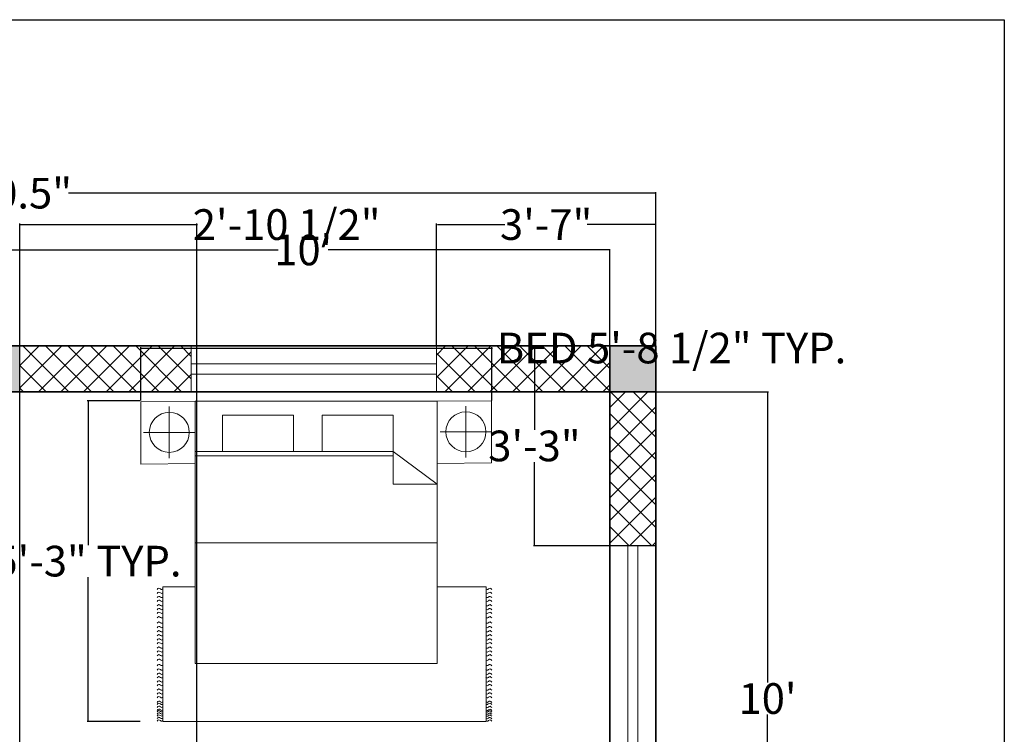
# Model space of a CAD drawing. Units: inches. Extents: x 958 to 1375, y 3152 to 3689.
# Tile 8 of 8: x 1182 to 1375, y 3550 to 3689. Entities that reach past the tile are written whole.
import ezdxf

# ---------------------------------------------------------------- set-up
doc = ezdxf.new("R2010")
doc.units = ezdxf.units.IN
doc.header["$MEASUREMENT"] = 0
for name, color, linetype, lineweight in [('A-ANNO-DIMS', 2, 'Continuous', 18), ('A-ANNO-TTLB', 7, 'Continuous', 25), ('A-FURN', 8, 'Continuous', 18), ('A-WALL', 7, 'Continuous', 35), ('windows', 140, 'Continuous', 18)]:
    doc.layers.add(name, color=color, linetype=linetype, lineweight=lineweight)
doc.layers.add('A-COLS-PATT', color=18, linetype='Continuous', lineweight=13, true_color=0x000000)
doc.layers.add('A-WALL-PATT', color=240, linetype='Continuous', lineweight=13, true_color=0xed1f24)
doc.styles.get("Standard").update_dxf_attribs({"font": 'arial.ttf'})
doc.dimstyles.get("Standard").update_dxf_attribs({"dimtxt": 6, "dimasz": 0.18, "dimexe": 0.18, "dimexo": 0.0625, "dimgap": 0.09, "dimtad": 0, "dimtih": 1, "dimtoh": 1, "dimdec": 1, "dimzin": 0, "dimdsep": 46, "dimlunit": 3, "dimtxsty": 'Standard', "dimcen": 0.09, "dimadec": 0, "dimazin": 0, "dimtfac": 1, "dimtdec": 1, "dimtofl": 0, "dimtmove": 0, "dimatfit": 3, "dimfxl": 1, "dimtolj": 1, "dimtzin": 0, "dimarcsym": 0})

# ---------------------------------------------------------------- blocks, each defined once
blk = doc.blocks.new('*D4')
at = {"layer": 'A-ANNO-DIMS', "color": 0, "lineweight": -2, "transparency": 16777216}
for p, q in [((1177.7, 3625.6), (1177.7, 3644.49)), ((1177.88, 3644.31), (1232.8, 3644.31)), ((1297.52, 3644.31), (1242.6, 3644.31)), ((1297.7, 3625.6), (1297.7, 3644.49))]:
    blk.add_line(p, q, dxfattribs=at)
at = {"layer": 'A-ANNO-DIMS', "color": 0, "transparency": 16777216}
for points in [[(1177.88, 3644.34), (1177.88, 3644.28), (1177.7, 3644.31)], [(1297.52, 3644.34), (1297.52, 3644.28), (1297.7, 3644.31)]]:
    blk.add_solid(points, dxfattribs=at)
at = {"layer": 'Defpoints', "color": 0, "transparency": 16777216}
for p in [(1297.7, 3644.31), (1177.7, 3625.53), (1297.7, 3625.53)]:
    blk.add_point(p, dxfattribs=at)
at = {"layer": 'A-ANNO-DIMS', "color": 0, "transparency": 16777216, "insert": (1237.7, 3644.31), "char_height": 6, "attachment_point": 5}
blk.add_mtext("\\A1;10'", dxfattribs=at)
blk = doc.blocks.new('*D5')
at = {"layer": 'A-ANNO-DIMS', "color": 0, "lineweight": -2, "transparency": 16777216}
for p, q in [((1306.76, 3616.53), (1328.75, 3616.53)), ((1328.57, 3616.35), (1328.57, 3559.69)), ((1328.57, 3496.71), (1328.57, 3553.38)), ((1306.76, 3496.53), (1328.75, 3496.53))]:
    blk.add_line(p, q, dxfattribs=at)
at = {"layer": 'A-ANNO-DIMS', "color": 0, "transparency": 16777216}
for points in [[(1328.54, 3616.35), (1328.6, 3616.35), (1328.57, 3616.53)], [(1328.54, 3496.71), (1328.6, 3496.71), (1328.57, 3496.53)]]:
    blk.add_solid(points, dxfattribs=at)
at = {"layer": 'Defpoints', "color": 0, "transparency": 16777216}
for p in [(1306.7, 3616.53), (1306.7, 3496.53), (1328.57, 3496.53)]:
    blk.add_point(p, dxfattribs=at)
at = {"layer": 'A-ANNO-DIMS', "color": 0, "transparency": 16777216, "insert": (1328.57, 3556.53), "char_height": 6, "attachment_point": 5}
blk.add_mtext("\\A1;10'", dxfattribs=at)
blk = doc.blocks.new('*D11')
at = {"layer": 'A-ANNO-DIMS', "color": 0, "lineweight": -2, "transparency": 16777216}
for p, q in [((1044.2, 3625.6), (1044.2, 3655.6)), ((1044.38, 3655.42), (1159.17, 3655.42)), ((1306.52, 3655.42), (1191.72, 3655.42)), ((1306.7, 3625.6), (1306.7, 3655.6))]:
    blk.add_line(p, q, dxfattribs=at)
at = {"layer": 'A-ANNO-DIMS', "color": 0, "transparency": 16777216}
for points in [[(1044.38, 3655.45), (1044.38, 3655.39), (1044.2, 3655.42)], [(1306.52, 3655.45), (1306.52, 3655.39), (1306.7, 3655.42)]]:
    blk.add_solid(points, dxfattribs=at)
at = {"layer": 'Defpoints', "color": 0, "transparency": 16777216}
for p in [(1306.7, 3655.42), (1044.2, 3625.53), (1306.7, 3625.53)]:
    blk.add_point(p, dxfattribs=at)
at = {"layer": 'A-ANNO-DIMS', "color": 0, "transparency": 16777216, "insert": (1175.45, 3655.42), "char_height": 6, "attachment_point": 5}
blk.add_mtext('\\A1;21\'-10.5"', dxfattribs=at)
blk = doc.blocks.new('BED-DOUBLE')
for p, q in [((63.65, 61.72), (63.65, 51.66)), ((5.6, 61.62), (5.6, 51.56)), ((10.63, 56.59), (0.57, 56.59)), ((68.68, 56.69), (58.62, 56.69)), ((49.39, 52.82), (10.63, 52.82)), ((49.39, 52.82), (58, 46.47)), ((49.44, 52.82), (49.44, 46.47)), ((49.44, 52), (10.63, 52)), ((49.44, 46.47), (58, 46.47)), ((58.05, 34.96), (10.63, 34.96)), ((4.36, 0), (4.36, 26.37)), ((4.36, 26.37), (10.65, 26.37)), ((58.05, 26.37), (67.59, 26.37)), ((67.59, 26.37), (67.59, 0)), ((67.59, 0), (4.36, 0))]:
    blk.add_line(p, q)
for points in [[(0, 50.39), (10.63, 50.5), (10.63, 62.68), (0, 62.58)], [(58.05, 62.68), (58.05, 11.37), (10.63, 11.37), (10.63, 62.68)], [(58.05, 50.5), (68.68, 50.6), (68.68, 62.78), (58.05, 62.68)], [(29.88, 59.98), (29.88, 52.82), (15.98, 52.82), (15.98, 59.98)], [(49.44, 59.98), (49.44, 52.82), (35.55, 52.82), (35.55, 59.98)]]:
    blk.add_lwpolyline(points, close=True)
for centre in [(5.6, 56.59), (63.65, 56.69)]:
    blk.add_circle(centre, 3.92)
for points, knots in [([(3.23, 25.84), (3.32, 25.96), (3.52, 26.2), (3.86, 25.96), (4.14, 25.78), (4.29, 25.89), (4.36, 25.94)], [0, 0, 0, 0, 0.400747, 0.791423, 1.067667, 1.29709, 1.29709, 1.29709, 1.29709]), ([(3.23, 25.06), (3.32, 25.18), (3.52, 25.42), (3.86, 25.18), (4.14, 25.01), (4.29, 25.11), (4.36, 25.16)], [0, 0, 0, 0, 0.400747, 0.791423, 1.067667, 1.29709, 1.29709, 1.29709, 1.29709]), ([(68.71, 25.84), (68.61, 25.96), (68.42, 26.2), (68.08, 25.96), (67.8, 25.78), (67.65, 25.89), (67.58, 25.94)], [0, 0, 0, 0, 0.400747, 0.791423, 1.067667, 1.29709, 1.29709, 1.29709, 1.29709]), ([(68.71, 25.06), (68.61, 25.18), (68.42, 25.42), (68.08, 25.18), (67.8, 25.01), (67.65, 25.11), (67.58, 25.16)], [0, 0, 0, 0, 0.400747, 0.791423, 1.067667, 1.29709, 1.29709, 1.29709, 1.29709]), ([(3.23, 24.24), (3.32, 24.36), (3.52, 24.6), (3.86, 24.36), (4.14, 24.19), (4.29, 24.3), (4.36, 24.34)], [0, 0, 0, 0, 0.400747, 0.791423, 1.067667, 1.29709, 1.29709, 1.29709, 1.29709]), ([(3.23, 23.51), (3.32, 23.63), (3.52, 23.87), (3.86, 23.63), (4.14, 23.46), (4.29, 23.57), (4.36, 23.62)], [0, 0, 0, 0, 0.400747, 0.791423, 1.067667, 1.29709, 1.29709, 1.29709, 1.29709]), ([(68.71, 24.24), (68.61, 24.36), (68.42, 24.6), (68.08, 24.36), (67.8, 24.19), (67.65, 24.3), (67.58, 24.34)], [0, 0, 0, 0, 0.400747, 0.791423, 1.067667, 1.29709, 1.29709, 1.29709, 1.29709]), ([(68.71, 23.51), (68.61, 23.63), (68.42, 23.87), (68.08, 23.63), (67.8, 23.46), (67.65, 23.57), (67.58, 23.62)], [0, 0, 0, 0, 0.400747, 0.791423, 1.067667, 1.29709, 1.29709, 1.29709, 1.29709]), ([(3.23, 22.63), (3.32, 22.75), (3.52, 22.99), (3.86, 22.75), (4.14, 22.58), (4.29, 22.69), (4.36, 22.73)], [0, 0, 0, 0, 0.400747, 0.791423, 1.067667, 1.29709, 1.29709, 1.29709, 1.29709]), ([(3.23, 21.88), (3.32, 22), (3.52, 22.24), (3.86, 22), (4.14, 21.83), (4.29, 21.93), (4.36, 21.98)], [0, 0, 0, 0, 0.400747, 0.791423, 1.067667, 1.29709, 1.29709, 1.29709, 1.29709]), ([(3.23, 21.15), (3.32, 21.27), (3.52, 21.51), (3.86, 21.27), (4.14, 21.1), (4.29, 21.21), (4.36, 21.25)], [0, 0, 0, 0, 0.400747, 0.791423, 1.067667, 1.29709, 1.29709, 1.29709, 1.29709]), ([(68.71, 22.63), (68.61, 22.75), (68.42, 22.99), (68.08, 22.75), (67.8, 22.58), (67.65, 22.69), (67.58, 22.73)], [0, 0, 0, 0, 0.400747, 0.791423, 1.067667, 1.29709, 1.29709, 1.29709, 1.29709]), ([(68.71, 21.88), (68.61, 22), (68.42, 22.24), (68.08, 22), (67.8, 21.83), (67.65, 21.93), (67.58, 21.98)], [0, 0, 0, 0, 0.400747, 0.791423, 1.067667, 1.29709, 1.29709, 1.29709, 1.29709]), ([(68.71, 21.15), (68.61, 21.27), (68.42, 21.51), (68.08, 21.27), (67.8, 21.1), (67.65, 21.21), (67.58, 21.25)], [0, 0, 0, 0, 0.400747, 0.791423, 1.067667, 1.29709, 1.29709, 1.29709, 1.29709]), ([(3.23, 20.27), (3.32, 20.39), (3.52, 20.63), (3.86, 20.39), (4.14, 20.22), (4.29, 20.32), (4.36, 20.37)], [0, 0, 0, 0, 0.400747, 0.791423, 1.067667, 1.29709, 1.29709, 1.29709, 1.29709]), ([(3.23, 19.23), (3.32, 19.35), (3.52, 19.59), (3.86, 19.35), (4.14, 19.18), (4.29, 19.29), (4.36, 19.33)], [0, 0, 0, 0, 0.400747, 0.791423, 1.067667, 1.29709, 1.29709, 1.29709, 1.29709]), ([(68.71, 20.27), (68.61, 20.39), (68.42, 20.63), (68.08, 20.39), (67.8, 20.22), (67.65, 20.32), (67.58, 20.37)], [0, 0, 0, 0, 0.400747, 0.791423, 1.067667, 1.29709, 1.29709, 1.29709, 1.29709]), ([(68.71, 19.23), (68.61, 19.35), (68.42, 19.59), (68.08, 19.35), (67.8, 19.18), (67.65, 19.29), (67.58, 19.33)], [0, 0, 0, 0, 0.400747, 0.791423, 1.067667, 1.29709, 1.29709, 1.29709, 1.29709]), ([(3.23, 18.35), (3.32, 18.47), (3.52, 18.71), (3.86, 18.47), (4.14, 18.3), (4.29, 18.4), (4.36, 18.45)], [0, 0, 0, 0, 0.400747, 0.791423, 1.067667, 1.29709, 1.29709, 1.29709, 1.29709]), ([(3.23, 17.53), (3.32, 17.65), (3.52, 17.89), (3.86, 17.65), (4.14, 17.48), (4.29, 17.59), (4.36, 17.64)], [0, 0, 0, 0, 0.400747, 0.791423, 1.067667, 1.29709, 1.29709, 1.29709, 1.29709]), ([(68.71, 18.35), (68.61, 18.47), (68.42, 18.71), (68.08, 18.47), (67.8, 18.3), (67.65, 18.4), (67.58, 18.45)], [0, 0, 0, 0, 0.400747, 0.791423, 1.067667, 1.29709, 1.29709, 1.29709, 1.29709]), ([(68.71, 17.53), (68.61, 17.65), (68.42, 17.89), (68.08, 17.65), (67.8, 17.48), (67.65, 17.59), (67.58, 17.64)], [0, 0, 0, 0, 0.400747, 0.791423, 1.067667, 1.29709, 1.29709, 1.29709, 1.29709]), ([(3.23, 16.76), (3.32, 16.88), (3.52, 17.12), (3.86, 16.88), (4.14, 16.71), (4.29, 16.81), (4.36, 16.86)], [0, 0, 0, 0, 0.400747, 0.791423, 1.067667, 1.29709, 1.29709, 1.29709, 1.29709]), ([(3.23, 15.94), (3.32, 16.06), (3.52, 16.3), (3.86, 16.06), (4.14, 15.89), (4.29, 16), (4.36, 16.04)], [0, 0, 0, 0, 0.400747, 0.791423, 1.067667, 1.29709, 1.29709, 1.29709, 1.29709]), ([(3.23, 15.21), (3.32, 15.33), (3.52, 15.57), (3.86, 15.33), (4.14, 15.16), (4.29, 15.27), (4.36, 15.32)], [0, 0, 0, 0, 0.400747, 0.791423, 1.067667, 1.29709, 1.29709, 1.29709, 1.29709]), ([(68.71, 16.76), (68.61, 16.88), (68.42, 17.12), (68.08, 16.88), (67.8, 16.71), (67.65, 16.81), (67.58, 16.86)], [0, 0, 0, 0, 0.400747, 0.791423, 1.067667, 1.29709, 1.29709, 1.29709, 1.29709]), ([(68.71, 15.94), (68.61, 16.06), (68.42, 16.3), (68.08, 16.06), (67.8, 15.89), (67.65, 16), (67.58, 16.04)], [0, 0, 0, 0, 0.400747, 0.791423, 1.067667, 1.29709, 1.29709, 1.29709, 1.29709]), ([(68.71, 15.21), (68.61, 15.33), (68.42, 15.57), (68.08, 15.33), (67.8, 15.16), (67.65, 15.27), (67.58, 15.32)], [0, 0, 0, 0, 0.400747, 0.791423, 1.067667, 1.29709, 1.29709, 1.29709, 1.29709]), ([(3.23, 14.33), (3.32, 14.45), (3.52, 14.69), (3.86, 14.45), (4.14, 14.28), (4.29, 14.39), (4.36, 14.43)], [0, 0, 0, 0, 0.400747, 0.791423, 1.067667, 1.29709, 1.29709, 1.29709, 1.29709]), ([(3.23, 13.58), (3.32, 13.7), (3.52, 13.94), (3.86, 13.7), (4.14, 13.53), (4.29, 13.63), (4.36, 13.68)], [0, 0, 0, 0, 0.400747, 0.791423, 1.067667, 1.29709, 1.29709, 1.29709, 1.29709]), ([(68.71, 14.33), (68.61, 14.45), (68.42, 14.69), (68.08, 14.45), (67.8, 14.28), (67.65, 14.39), (67.58, 14.43)], [0, 0, 0, 0, 0.400747, 0.791423, 1.067667, 1.29709, 1.29709, 1.29709, 1.29709]), ([(68.71, 13.58), (68.61, 13.7), (68.42, 13.94), (68.08, 13.7), (67.8, 13.53), (67.65, 13.63), (67.58, 13.68)], [0, 0, 0, 0, 0.400747, 0.791423, 1.067667, 1.29709, 1.29709, 1.29709, 1.29709]), ([(3.23, 12.85), (3.32, 12.97), (3.52, 13.21), (3.86, 12.97), (4.14, 12.8), (4.29, 12.9), (4.36, 12.95)], [0, 0, 0, 0, 0.400747, 0.791423, 1.067667, 1.29709, 1.29709, 1.29709, 1.29709]), ([(3.23, 11.97), (3.32, 12.09), (3.52, 12.33), (3.86, 12.09), (4.14, 11.92), (4.29, 12.02), (4.36, 12.07)], [0, 0, 0, 0, 0.400747, 0.791423, 1.067667, 1.29709, 1.29709, 1.29709, 1.29709]), ([(68.71, 12.85), (68.61, 12.97), (68.42, 13.21), (68.08, 12.97), (67.8, 12.8), (67.65, 12.9), (67.58, 12.95)], [0, 0, 0, 0, 0.400747, 0.791423, 1.067667, 1.29709, 1.29709, 1.29709, 1.29709]), ([(68.71, 11.97), (68.61, 12.09), (68.42, 12.33), (68.08, 12.09), (67.8, 11.92), (67.65, 12.02), (67.58, 12.07)], [0, 0, 0, 0, 0.400747, 0.791423, 1.067667, 1.29709, 1.29709, 1.29709, 1.29709]), ([(3.23, 10.93), (3.32, 11.05), (3.52, 11.29), (3.86, 11.05), (4.14, 10.88), (4.29, 10.99), (4.36, 11.03)], [0, 0, 0, 0, 0.400747, 0.791423, 1.067667, 1.29709, 1.29709, 1.29709, 1.29709]), ([(3.23, 10.05), (3.32, 10.17), (3.52, 10.41), (3.86, 10.17), (4.14, 10), (4.29, 10.1), (4.36, 10.15)], [0, 0, 0, 0, 0.400747, 0.791423, 1.067667, 1.29709, 1.29709, 1.29709, 1.29709]), ([(68.71, 10.93), (68.61, 11.05), (68.42, 11.29), (68.08, 11.05), (67.8, 10.88), (67.65, 10.99), (67.58, 11.03)], [0, 0, 0, 0, 0.400747, 0.791423, 1.067667, 1.29709, 1.29709, 1.29709, 1.29709]), ([(68.71, 10.05), (68.61, 10.17), (68.42, 10.41), (68.08, 10.17), (67.8, 10), (67.65, 10.1), (67.58, 10.15)], [0, 0, 0, 0, 0.400747, 0.791423, 1.067667, 1.29709, 1.29709, 1.29709, 1.29709]), ([(3.23, 9.23), (3.32, 9.35), (3.52, 9.59), (3.86, 9.35), (4.14, 9.18), (4.29, 9.29), (4.36, 9.34)], [0, 0, 0, 0, 0.400747, 0.791423, 1.067667, 1.29709, 1.29709, 1.29709, 1.29709]), ([(3.23, 8.54), (3.32, 8.66), (3.52, 8.9), (3.86, 8.66), (4.14, 8.49), (4.29, 8.6), (4.36, 8.65)], [0, 0, 0, 0, 0.400747, 0.791423, 1.067667, 1.29709, 1.29709, 1.29709, 1.29709]), ([(3.23, 7.73), (3.32, 7.85), (3.52, 8.09), (3.86, 7.85), (4.14, 7.68), (4.29, 7.78), (4.36, 7.83)], [0, 0, 0, 0, 0.400747, 0.791423, 1.067667, 1.29709, 1.29709, 1.29709, 1.29709]), ([(68.71, 9.23), (68.61, 9.35), (68.42, 9.59), (68.08, 9.35), (67.8, 9.18), (67.65, 9.29), (67.58, 9.34)], [0, 0, 0, 0, 0.400747, 0.791423, 1.067667, 1.29709, 1.29709, 1.29709, 1.29709]), ([(68.71, 8.54), (68.61, 8.66), (68.42, 8.9), (68.08, 8.66), (67.8, 8.49), (67.65, 8.6), (67.58, 8.65)], [0, 0, 0, 0, 0.400747, 0.791423, 1.067667, 1.29709, 1.29709, 1.29709, 1.29709]), ([(68.71, 7.73), (68.61, 7.85), (68.42, 8.09), (68.08, 7.85), (67.8, 7.68), (67.65, 7.78), (67.58, 7.83)], [0, 0, 0, 0, 0.400747, 0.791423, 1.067667, 1.29709, 1.29709, 1.29709, 1.29709]), ([(3.23, 7), (3.32, 7.12), (3.52, 7.36), (3.86, 7.12), (4.14, 6.95), (4.29, 7.05), (4.36, 7.1)], [0, 0, 0, 0, 0.400747, 0.791423, 1.067667, 1.29709, 1.29709, 1.29709, 1.29709]), ([(3.23, 6.12), (3.32, 6.24), (3.52, 6.48), (3.86, 6.24), (4.14, 6.07), (4.29, 6.17), (4.36, 6.22)], [0, 0, 0, 0, 0.400747, 0.791423, 1.067667, 1.29709, 1.29709, 1.29709, 1.29709]), ([(68.71, 7), (68.61, 7.12), (68.42, 7.36), (68.08, 7.12), (67.8, 6.95), (67.65, 7.05), (67.58, 7.1)], [0, 0, 0, 0, 0.400747, 0.791423, 1.067667, 1.29709, 1.29709, 1.29709, 1.29709]), ([(68.71, 6.12), (68.61, 6.24), (68.42, 6.48), (68.08, 6.24), (67.8, 6.07), (67.65, 6.17), (67.58, 6.22)], [0, 0, 0, 0, 0.400747, 0.791423, 1.067667, 1.29709, 1.29709, 1.29709, 1.29709]), ([(3.23, 5.37), (3.32, 5.49), (3.52, 5.73), (3.86, 5.49), (4.14, 5.31), (4.29, 5.42), (4.36, 5.47)], [0, 0, 0, 0, 0.400747, 0.791423, 1.067667, 1.29709, 1.29709, 1.29709, 1.29709]), ([(3.23, 4.64), (3.32, 4.76), (3.52, 5), (3.86, 4.76), (4.14, 4.59), (4.29, 4.69), (4.36, 4.74)], [0, 0, 0, 0, 0.400747, 0.791423, 1.067667, 1.29709, 1.29709, 1.29709, 1.29709]), ([(3.23, 3.75), (3.32, 3.88), (3.52, 4.12), (3.86, 3.88), (4.14, 3.7), (4.29, 3.81), (4.36, 3.86)], [0, 0, 0, 0, 0.400747, 0.791423, 1.067667, 1.29709, 1.29709, 1.29709, 1.29709]), ([(68.71, 5.37), (68.61, 5.49), (68.42, 5.73), (68.08, 5.49), (67.8, 5.31), (67.65, 5.42), (67.58, 5.47)], [0, 0, 0, 0, 0.400747, 0.791423, 1.067667, 1.29709, 1.29709, 1.29709, 1.29709]), ([(68.71, 4.64), (68.61, 4.76), (68.42, 5), (68.08, 4.76), (67.8, 4.59), (67.66, 4.69), (67.59, 4.73)], [0, 0, 0, 0, 0.400747, 0.791423, 1.067667, 1.283686, 1.283686, 1.283686, 1.283686]), ([(68.71, 3.75), (68.61, 3.88), (68.42, 4.12), (68.08, 3.88), (67.8, 3.7), (67.66, 3.81), (67.59, 3.85)], [0, 0, 0, 0, 0.400747, 0.791423, 1.067667, 1.283686, 1.283686, 1.283686, 1.283686]), ([(3.23, 3.33), (3.32, 3.45), (3.52, 3.7), (3.86, 3.45), (4.14, 3.27), (4.29, 3.38), (4.36, 3.43)], [0, 0, 0, 0, 0.407265, 0.802015, 1.07826, 1.307683, 1.307683, 1.307683, 1.307683]), ([(3.23, 2.76), (3.32, 2.88), (3.52, 3.12), (3.86, 2.88), (4.14, 2.71), (4.29, 2.81), (4.36, 2.86)], [0, 0, 0, 0, 0.400747, 0.791423, 1.067667, 1.29709, 1.29709, 1.29709, 1.29709]), ([(3.23, 2.19), (3.32, 2.31), (3.52, 2.55), (3.86, 2.31), (4.14, 2.13), (4.29, 2.24), (4.36, 2.29)], [0, 0, 0, 0, 0.400747, 0.791423, 1.067667, 1.29709, 1.29709, 1.29709, 1.29709]), ([(3.23, 1.88), (3.32, 2), (3.52, 2.24), (3.86, 2), (4.14, 1.82), (4.29, 1.93), (4.36, 1.98)], [0, 0, 0, 0, 0.400747, 0.791423, 1.067667, 1.29709, 1.29709, 1.29709, 1.29709]), ([(68.71, 3.33), (68.61, 3.45), (68.42, 3.69), (68.08, 3.45), (67.8, 3.28), (67.66, 3.38), (67.59, 3.42)], [0, 0, 0, 0, 0.402903, 0.794912, 1.071156, 1.287177, 1.287177, 1.287177, 1.287177]), ([(68.71, 2.73), (68.61, 2.85), (68.42, 3.09), (68.08, 2.85), (67.8, 2.68), (67.66, 2.78), (67.59, 2.83)], [0, 0, 0, 0, 0.400747, 0.791423, 1.067667, 1.283686, 1.283686, 1.283686, 1.283686]), ([(68.71, 2.16), (68.61, 2.28), (68.42, 2.52), (68.08, 2.28), (67.8, 2.11), (67.66, 2.21), (67.59, 2.25)], [0, 0, 0, 0, 0.400747, 0.791423, 1.067667, 1.283686, 1.283686, 1.283686, 1.283686]), ([(68.71, 1.85), (68.61, 1.97), (68.42, 2.21), (68.08, 1.97), (67.8, 1.8), (67.66, 1.9), (67.59, 1.94)], [0, 0, 0, 0, 0.400747, 0.791423, 1.067667, 1.283686, 1.283686, 1.283686, 1.283686]), ([(3.23, 1.46), (3.32, 1.58), (3.52, 1.82), (3.86, 1.58), (4.14, 1.41), (4.29, 1.51), (4.36, 1.56)], [0, 0, 0, 0, 0.400747, 0.791423, 1.067667, 1.29709, 1.29709, 1.29709, 1.29709]), ([(3.23, 1.06), (3.32, 1.18), (3.52, 1.42), (3.86, 1.18), (4.14, 1.01), (4.29, 1.11), (4.36, 1.16)], [0, 0, 0, 0, 0.400747, 0.791423, 1.067667, 1.29709, 1.29709, 1.29709, 1.29709]), ([(3.23, 0.57), (3.32, 0.7), (3.52, 0.94), (3.86, 0.7), (4.14, 0.52), (4.29, 0.63), (4.36, 0.68)], [0, 0, 0, 0, 0.400747, 0.791423, 1.067667, 1.29709, 1.29709, 1.29709, 1.29709]), ([(3.23, 0.07), (3.32, 0.19), (3.52, 0.43), (3.86, 0.19), (4.14, 0.02), (4.29, 0.13), (4.36, 0.18)], [0, 0, 0, 0, 0.400747, 0.791423, 1.067667, 1.29709, 1.29709, 1.29709, 1.29709]), ([(68.71, 1.43), (68.61, 1.55), (68.42, 1.79), (68.08, 1.55), (67.8, 1.38), (67.65, 1.48), (67.58, 1.53)], [0, 0, 0, 0, 0.400747, 0.791423, 1.067667, 1.29709, 1.29709, 1.29709, 1.29709]), ([(68.71, 1.03), (68.61, 1.15), (68.42, 1.39), (68.08, 1.15), (67.8, 0.98), (67.65, 1.09), (67.58, 1.13)], [0, 0, 0, 0, 0.400747, 0.791423, 1.067667, 1.29709, 1.29709, 1.29709, 1.29709]), ([(68.71, 0.55), (68.61, 0.67), (68.42, 0.91), (68.08, 0.67), (67.8, 0.5), (67.65, 0.6), (67.58, 0.65)], [0, 0, 0, 0, 0.400747, 0.791423, 1.067667, 1.29709, 1.29709, 1.29709, 1.29709]), ([(68.71, 0.07), (68.61, 0.19), (68.42, 0.43), (68.08, 0.19), (67.8, 0.02), (67.65, 0.13), (67.58, 0.18)], [0, 0, 0, 0, 0.400747, 0.791423, 1.067667, 1.29709, 1.29709, 1.29709, 1.29709])]:
    blk.add_open_spline(points, degree=3, knots=knots)
blk = doc.blocks.new('WIN-48')
for p, q in [((48, 9), (0, 9)), ((48, 5.5), (0, 5.5)), ((0, 3.5), (48, 3.5)), ((0, 0), (48, 0))]:
    blk.add_line(p, q)
blk = doc.blocks.new('*D26')
at = {"layer": 'A-ANNO-DIMS', "color": 0, "lineweight": -2, "transparency": 16777216}
for p, q in [((1205.88, 3614.87), (1205.88, 3625.3)), ((1206.06, 3625.12), (1274.41, 3625.12)), ((1274.59, 3614.87), (1274.59, 3625.3)), ((1274.59, 3625.12), (1274.77, 3625.12))]:
    blk.add_line(p, q, dxfattribs=at)
at = {"layer": 'A-ANNO-DIMS', "color": 0, "transparency": 16777216}
for points in [[(1206.06, 3625.15), (1206.06, 3625.09), (1205.88, 3625.12)], [(1274.41, 3625.15), (1274.41, 3625.09), (1274.59, 3625.12)]]:
    blk.add_solid(points, dxfattribs=at)
at = {"layer": 'Defpoints', "color": 0, "transparency": 16777216}
for p in [(1274.59, 3625.12), (1205.88, 3614.81), (1274.59, 3614.81)]:
    blk.add_point(p, dxfattribs=at)
at = {"layer": 'A-ANNO-DIMS', "color": 0, "transparency": 16777216, "insert": (1309.78, 3625.12), "char_height": 6, "attachment_point": 5}
blk.add_mtext('\\A1;BED 5\'-8 1/2" TYP.', dxfattribs=at)
blk = doc.blocks.new('*D27')
at = {"layer": 'A-ANNO-DIMS', "color": 0, "lineweight": -2, "transparency": 16777216}
for p, q in [((1205.81, 3614.81), (1195.39, 3614.81)), ((1195.57, 3614.63), (1195.57, 3586.57)), ((1195.57, 3552.21), (1195.57, 3580.26)), ((1205.81, 3552.03), (1195.39, 3552.03))]:
    blk.add_line(p, q, dxfattribs=at)
at = {"layer": 'A-ANNO-DIMS', "color": 0, "transparency": 16777216}
for points in [[(1195.54, 3614.63), (1195.6, 3614.63), (1195.57, 3614.81)], [(1195.54, 3552.21), (1195.6, 3552.21), (1195.57, 3552.03)]]:
    blk.add_solid(points, dxfattribs=at)
at = {"layer": 'Defpoints', "color": 0, "transparency": 16777216}
for p in [(1195.57, 3614.81), (1205.88, 3614.81), (1205.88, 3552.03)]:
    blk.add_point(p, dxfattribs=at)
at = {"layer": 'A-ANNO-DIMS', "color": 0, "transparency": 16777216, "insert": (1195.57, 3583.42), "char_height": 6, "attachment_point": 5}
blk.add_mtext('\\A1;5\'-3" TYP.', dxfattribs=at)
blk = doc.blocks.new('*D47')
at = {"layer": 'A-ANNO-DIMS', "color": 0, "lineweight": -2, "transparency": 16777216}
for p, q in [((1182.2, 3492.1), (1182.2, 3649.46)), ((1182.38, 3649.28), (1216.66, 3649.28)), ((1216.84, 3496.6), (1216.84, 3649.46)), ((1216.84, 3649.28), (1217.02, 3649.28))]:
    blk.add_line(p, q, dxfattribs=at)
at = {"layer": 'A-ANNO-DIMS', "color": 0, "transparency": 16777216}
for points in [[(1182.38, 3649.31), (1182.38, 3649.25), (1182.2, 3649.28)], [(1216.66, 3649.31), (1216.66, 3649.25), (1216.84, 3649.28)]]:
    blk.add_solid(points, dxfattribs=at)
at = {"layer": 'Defpoints', "color": 0, "transparency": 16777216}
for p in [(1216.84, 3649.28), (1216.84, 3496.53), (1182.2, 3492.03)]:
    blk.add_point(p, dxfattribs=at)
at = {"layer": 'A-ANNO-DIMS', "color": 0, "transparency": 16777216, "insert": (1234.45, 3649.28), "char_height": 6, "attachment_point": 5}
blk.add_mtext('\\A1;2\'-10 1/2"', dxfattribs=at)
blk = doc.blocks.new('*D51')
at = {"layer": 'A-ANNO-DIMS', "color": 0, "lineweight": -2, "transparency": 16777216}
for p, q in [((1263.78, 3625.6), (1263.78, 3649.46)), ((1263.96, 3649.28), (1277.17, 3649.28)), ((1306.52, 3649.28), (1293.3, 3649.28)), ((1306.7, 3625.6), (1306.7, 3649.46))]:
    blk.add_line(p, q, dxfattribs=at)
at = {"layer": 'A-ANNO-DIMS', "color": 0, "transparency": 16777216}
for points in [[(1263.96, 3649.31), (1263.96, 3649.25), (1263.78, 3649.28)], [(1306.52, 3649.31), (1306.52, 3649.25), (1306.7, 3649.28)]]:
    blk.add_solid(points, dxfattribs=at)
at = {"layer": 'Defpoints', "color": 0, "transparency": 16777216}
for p in [(1306.7, 3649.28), (1263.78, 3625.53), (1306.7, 3625.53)]:
    blk.add_point(p, dxfattribs=at)
at = {"layer": 'A-ANNO-DIMS', "color": 0, "transparency": 16777216, "insert": (1285.24, 3649.28), "char_height": 6, "attachment_point": 5}
blk.add_mtext('\\A1;3\'-7"', dxfattribs=at)
blk = doc.blocks.new('*D53')
at = {"layer": 'A-ANNO-DIMS', "color": 0, "lineweight": -2, "transparency": 16777216}
for p, q in [((1306.63, 3625.53), (1282.77, 3625.53)), ((1282.95, 3625.35), (1282.95, 3609.11)), ((1282.95, 3586.56), (1282.95, 3602.8)), ((1306.63, 3586.38), (1282.77, 3586.38))]:
    blk.add_line(p, q, dxfattribs=at)
at = {"layer": 'A-ANNO-DIMS', "color": 0, "transparency": 16777216}
for points in [[(1282.92, 3625.35), (1282.98, 3625.35), (1282.95, 3625.53)], [(1282.92, 3586.56), (1282.98, 3586.56), (1282.95, 3586.38)]]:
    blk.add_solid(points, dxfattribs=at)
at = {"layer": 'Defpoints', "color": 0, "transparency": 16777216}
for p in [(1282.95, 3625.53), (1306.7, 3625.53), (1306.7, 3586.38)]:
    blk.add_point(p, dxfattribs=at)
at = {"layer": 'A-ANNO-DIMS', "color": 0, "transparency": 16777216, "insert": (1282.95, 3605.96), "char_height": 6, "attachment_point": 5}
blk.add_mtext('\\A1;3\'-3"', dxfattribs=at)

msp = doc.modelspace()

# ---------------------------------------------------------------- hatches: boundary and pattern name
at = {"layer": 'A-COLS-PATT'}
h = msp.add_hatch(color=256, dxfattribs=at)
h.dxf.hatch_style = 1
h.paths.add_polyline_path([(1053.2, 3625.53), (1044.2, 3625.53), (1044.2, 3616.53), (1053.2, 3616.53)])
h.paths.add_polyline_path([(1182.2, 3625.53), (1173.2, 3625.53), (1173.2, 3616.53), (1182.2, 3616.53)])
h.paths.add_polyline_path([(1306.7, 3625.53), (1297.7, 3625.53), (1297.7, 3616.53), (1306.7, 3616.53)])
h.paths.add_polyline_path([(1306.7, 3501.03), (1297.7, 3501.03), (1297.7, 3492.03), (1306.7, 3492.03)])
h.paths.add_polyline_path([(1306.7, 3391.53), (1297.7, 3391.53), (1297.7, 3382.53), (1306.7, 3382.53)])
h.paths.add_polyline_path([(1306.7, 3267.03), (1297.7, 3267.03), (1297.7, 3258.03), (1306.7, 3258.03)])
h.paths.add_polyline_path([(1182.2, 3267.03), (1173.2, 3267.03), (1173.2, 3258.03), (1182.2, 3258.03)])
h.paths.add_polyline_path([(1053.2, 3267.03), (1044.2, 3267.03), (1044.2, 3258.03), (1053.2, 3258.03)])
h.paths.add_polyline_path([(1053.2, 3391.53), (1044.2, 3391.53), (1044.2, 3382.53), (1053.2, 3382.53)])
h.paths.add_polyline_path([(1053.2, 3501.03), (1044.2, 3501.03), (1044.2, 3492.03), (1053.2, 3492.03)])
h.paths.add_polyline_path([(1182.2, 3501.03), (1173.2, 3501.03), (1173.2, 3492.03), (1182.2, 3492.03)])
h.paths.add_polyline_path([(1182.2, 3391.53), (1173.2, 3391.53), (1173.2, 3382.53), (1182.2, 3382.53)])
at = {"layer": 'A-WALL-PATT'}
h = msp.add_hatch(dxfattribs=at)
h.set_pattern_fill('ANSI37', color=256, scale=25)
h.paths.add_polyline_path([(1080.68, 3625.53), (1053.2, 3625.53), (1053.2, 3616.53), (1080.68, 3616.53)])
h.paths.add_polyline_path([(1053.2, 3616.53), (1044.2, 3616.53), (1044.2, 3587.05), (1053.2, 3587.05)])
h.paths.add_polyline_path([(1173.2, 3625.53), (1128.68, 3625.53), (1128.68, 3616.53), (1173.2, 3616.53)])
h.paths.add_polyline_path([(1215.78, 3625.53), (1182.2, 3625.53), (1182.2, 3616.53), (1215.78, 3616.53)])
h.paths.add_polyline_path([(1297.7, 3625.53), (1263.78, 3625.53), (1263.78, 3616.53), (1297.7, 3616.53)])
h.paths.add_polyline_path([(1177.7, 3616.53), (1173.2, 3616.53), (1173.2, 3501.03), (1177.7, 3501.03)])
h.paths.add_polyline_path([(1053.2, 3539.05), (1044.2, 3539.05), (1044.2, 3501.03), (1053.2, 3501.03)])
h.paths.add_polyline_path([(1135.44, 3496.53), (1053.2, 3496.53), (1053.2, 3492.03), (1135.44, 3492.03)])
h.paths.add_polyline_path([(1306.7, 3616.53), (1297.7, 3616.53), (1297.7, 3586.38), (1306.7, 3586.38)])
h.paths.add_polyline_path([(1306.7, 3538.38), (1297.7, 3538.38), (1297.7, 3501.03), (1306.7, 3501.03)])
h.paths.add_polyline_path([(1297.7, 3496.53), (1216.84, 3496.53), (1216.84, 3492.03), (1297.7, 3492.03)])
h.paths.add_polyline_path([(1306.7, 3492.03), (1297.7, 3492.03), (1297.7, 3481.63), (1306.7, 3481.63)])
h.paths.add_polyline_path([(1306.7, 3457.63), (1297.7, 3457.63), (1297.7, 3444.03), (1225.7, 3444.03), (1225.7, 3462.51), (1221.2, 3462.51), (1221.2, 3391.53), (1182.2, 3391.53), (1182.2, 3387.03), (1225.7, 3387.03), (1225.7, 3439.53), (1297.7, 3439.53), (1297.7, 3428.57), (1306.7, 3428.57)])
h.paths.add_polyline_path([(1306.7, 3404.57), (1297.7, 3404.57), (1297.7, 3391.53), (1306.7, 3391.53)], flags=17)
h.paths.add_polyline_path([(1297.7, 3391.53), (1253.12, 3391.53), (1253.12, 3387.03), (1297.7, 3387.03)], flags=17)
h.paths.add_polyline_path([(1306.7, 3382.53), (1297.7, 3382.53), (1297.7, 3354.01), (1306.7, 3354.01)])
h.paths.add_polyline_path([(1306.7, 3306.01), (1297.7, 3306.01), (1297.7, 3267.03), (1306.7, 3267.03)])
h.paths.add_polyline_path([(1297.7, 3267.03), (1254.05, 3267.03), (1254.05, 3258.03), (1297.7, 3258.03)])
h.paths.add_polyline_path([(1177.7, 3347.74), (1173.2, 3347.74), (1173.2, 3267.03), (1177.7, 3267.03)])
h.paths.add_polyline_path([(1206.05, 3267.03), (1182.2, 3267.03), (1182.2, 3258.03), (1206.05, 3258.03)])
h.paths.add_polyline_path([(1053.2, 3308.96), (1044.2, 3308.96), (1044.2, 3267.03), (1053.2, 3267.03)])
h.paths.add_polyline_path([(1053.2, 3382.53), (1044.2, 3382.53), (1044.2, 3356.96), (1053.2, 3356.96)])
h.paths.add_polyline_path([(1053.2, 3420.58), (1044.2, 3420.58), (1044.2, 3391.53), (1053.2, 3391.53)])
h.paths.add_polyline_path([(1053.2, 3492.03), (1044.2, 3492.03), (1044.2, 3468.58), (1053.2, 3468.58)])

# ---------------------------------------------------------------- linework, layer by layer
at = {"layer": 'A-ANNO-TTLB'}
msp.add_lwpolyline([(958.44, 3689.37), (1374.91, 3689.37), (1374.91, 3152.28), (958.44, 3152.28)], close=True, dxfattribs=at)
at = {"layer": 'A-WALL'}
for p, q in [((1044.2, 3625.53), (1306.7, 3625.53)), ((1297.7, 3625.53), (1297.7, 3444.03)), ((1306.7, 3625.53), (1306.7, 3258.03)), ((1044.2, 3616.53), (1306.7, 3616.53))]:
    msp.add_line(p, q, dxfattribs=at)
at = {"layer": 'windows'}
for p, q in [((1215.78, 3625.53), (1215.78, 3616.53)), ((1263.78, 3616.53), (1263.78, 3625.53)), ((1297.7, 3586.38), (1306.7, 3586.38))]:
    msp.add_line(p, q, dxfattribs=at)

# ---------------------------------------------------------------- block references
at = {"layer": 'A-FURN'}
msp.add_blockref('BED-DOUBLE', (1205.88, 3552.03), dxfattribs=at)
at = {"layer": 'windows'}
msp.add_blockref('WIN-48', (1215.78, 3616.53), dxfattribs=at)
at = {"layer": 'windows', "rotation": 90}
msp.add_blockref('WIN-48', (1306.7, 3538.38), dxfattribs=at)

# ---------------------------------------------------------------- dimensions: what is measured, and where the dimension line sits
at = {"layer": 'A-ANNO-DIMS'}
for base, p1, p2, override, picture, middle in [((1306.7, 3655.42), (1044.2, 3625.53), (1306.7, 3625.53), {"dimclrd": 0, "dimclre": 0, "dimclrt": 0}, '*D11', (1175.45, 3655.42)), ((1216.84, 3649.28), (1182.2, 3492.03), (1216.84, 3496.53), {"dimdec": 1, "dimlfac": 1, "dimrnd": 0, "dimzin": 1, "dimdsep": 46, "dimlunit": 4, "dimfrac": 2}, '*D47', (1234.45, 3649.28)), ((1297.7, 3644.31), (1177.7, 3625.53), (1297.7, 3625.53), {"dimclrd": 0, "dimclre": 0, "dimclrt": 0}, '*D4', (1237.7, 3644.31))]:
    dim = msp.add_linear_dim(base=base, p1=p1, p2=p2, dimstyle='Standard', override=override, dxfattribs=at)
    dim.commit()
    dim.dimension.update_dxf_attribs({"geometry": picture, "text_midpoint": middle})
for base, p1, p2, angle, override, picture, middle in [((1306.7, 3649.28), (1263.78, 3625.53), (1306.7, 3625.53), 0, {"dimdec": 1, "dimlfac": 1, "dimrnd": 0, "dimzin": 1, "dimdsep": 46, "dimlunit": 4, "dimfrac": 2}, '*D51', (1285.24, 3649.28)), ((1282.9472, 3625.5349), (1306.6972, 3586.3802), (1306.6972, 3625.5349), 90, {"dimdec": 1, "dimlfac": 1, "dimrnd": 0, "dimzin": 1, "dimdsep": 46, "dimlunit": 4, "dimfrac": 2}, '*D53', (1282.9472, 3605.9576)), ((1328.57, 3496.53), (1306.7, 3616.53), (1306.7, 3496.53), 90, {"dimclrd": 0, "dimclre": 0, "dimclrt": 0}, '*D5', (1328.57, 3556.53))]:
    dim = msp.add_linear_dim(base=base, p1=p1, p2=p2, angle=angle, dimstyle='Standard', override=override, dxfattribs=at)
    dim.commit()
    dim.dimension.update_dxf_attribs({"geometry": picture, "text_midpoint": middle})
dim = msp.add_linear_dim(base=(1274.59, 3625.12), p1=(1205.88, 3614.81), p2=(1274.59, 3614.81), text='BED <> TYP.', dimstyle='Standard', override={"dimdec": 1, "dimlfac": 1, "dimrnd": 0, "dimzin": 1, "dimdsep": 46, "dimlunit": 4, "dimfrac": 2}, dxfattribs=at)
dim.commit()
dim.dimension.update_dxf_attribs({"geometry": '*D26', "text_midpoint": (1309.78, 3625.12)})
dim = msp.add_linear_dim(base=(1195.57, 3614.81), p1=(1205.88, 3552.03), p2=(1205.88, 3614.81), angle=90, text='<> TYP.', dimstyle='Standard', override={"dimdec": 1, "dimlfac": 1, "dimrnd": 0, "dimzin": 1, "dimdsep": 46, "dimlunit": 4, "dimfrac": 2}, dxfattribs=at)
dim.commit()
dim.dimension.update_dxf_attribs({"geometry": '*D27', "text_midpoint": (1195.57, 3583.42)})

doc.saveas('drawing.dxf')
